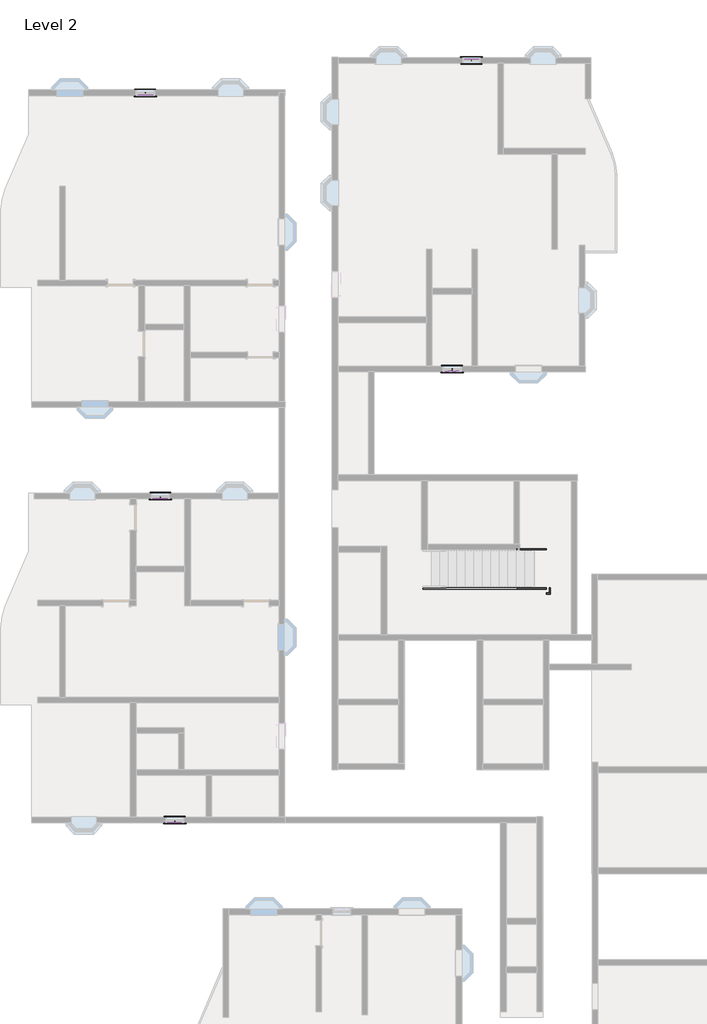
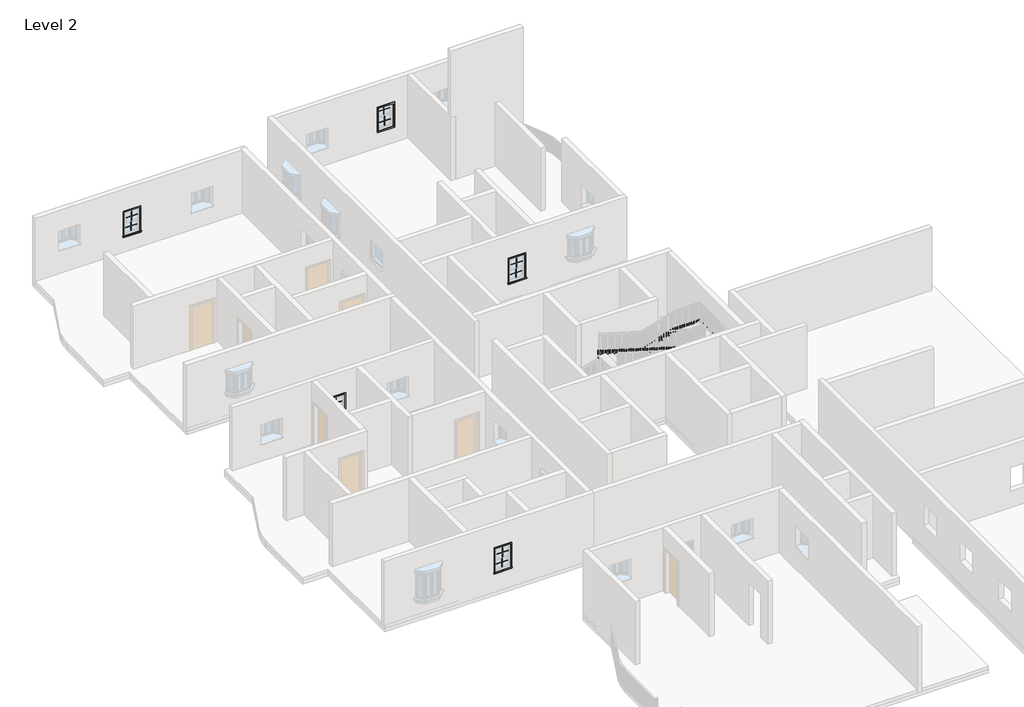
# One storey, part 14 of 14: 20 proxies, 6 members.
"""IFC4 building model written with IfcOpenShell, lengths in millimetres."""

from ifc_helpers import new_model, si_unit, frame, origin, place, context, project, spatial, polyline, outline, extrude, transform, mapped, element, save
from components import muntin_pattern_2x2_muntin_pattern_2x2_c35c595f, trim_window_exterior_flat_with_sill_e38017c9, trim_window_interior_flat_picture_frame_d728ed12

model = new_model("IFC4")

# Units and contexts
model_context = context("Model", 3, world=origin())
ifc_project = project(units=[si_unit("LENGTHUNIT", "METRE", prefix="MILLI")], contexts=[model_context])

# Site, building, storey
site = spatial("IfcSite", under=ifc_project)
building = spatial("IfcBuilding", under=site)
storey = spatial("IfcBuildingStorey", under=building, Name="Level 2", Elevation=3048.0)

# Proxies
placement = place(None, origin())
muntin_pattern_2x2_muntin_pattern_2x2_shape = muntin_pattern_2x2_muntin_pattern_2x2_c35c595f(model_context)
element("IfcBuildingElementProxy", 1, Name="Muntin Pattern_2x2 : Muntin Pattern_2x2", ObjectType="Muntin Pattern_2x2 : Muntin Pattern_2x2", at=placement, inside=storey, context=model_context, shape_type="MappedRepresentation", body=[
    mapped(muntin_pattern_2x2_muntin_pattern_2x2_shape, transform((-14639.3891351, 14368.0833494, 4518.025), x_axis=(-1.0, 0.0, 0.0), y_axis=(0.0, -1.0, 0.0), z_axis=(0.0, 0.0, 1.0))),
])
element("IfcBuildingElementProxy", 2, Name="Muntin Pattern_2x2 : Muntin Pattern_2x2", ObjectType="Muntin Pattern_2x2 : Muntin Pattern_2x2", at=placement, inside=storey, context=model_context, shape_type="MappedRepresentation", body=[
    mapped(muntin_pattern_2x2_muntin_pattern_2x2_shape, transform((-14639.3891351, 14412.5333494, 4038.6), x_axis=(-1.0, 0.0, 0.0), y_axis=(0.0, -1.0, 0.0), z_axis=(0.0, 0.0, 1.0))),
])
element("IfcBuildingElementProxy", 3, Name="Muntin Pattern_2x2 : Muntin Pattern_2x2", ObjectType="Muntin Pattern_2x2 : Muntin Pattern_2x2", at=placement, inside=storey, context=model_context, shape_type="MappedRepresentation", body=[
    mapped(muntin_pattern_2x2_muntin_pattern_2x2_shape, transform((-14125.0391351, 2785.6833494, 4518.025), x_axis=(-1.0, 0.0, 0.0), y_axis=(0.0, -1.0, 0.0), z_axis=(0.0, 0.0, 1.0))),
])
element("IfcBuildingElementProxy", 4, Name="Muntin Pattern_2x2 : Muntin Pattern_2x2", ObjectType="Muntin Pattern_2x2 : Muntin Pattern_2x2", at=placement, inside=storey, context=model_context, shape_type="MappedRepresentation", body=[
    mapped(muntin_pattern_2x2_muntin_pattern_2x2_shape, transform((-14125.0391351, 2830.1333494, 4038.6), x_axis=(-1.0, 0.0, 0.0), y_axis=(0.0, -1.0, 0.0), z_axis=(0.0, 0.0, 1.0))),
])
element("IfcBuildingElementProxy", 5, Name="Muntin Pattern_2x2 : Muntin Pattern_2x2", ObjectType="Muntin Pattern_2x2 : Muntin Pattern_2x2", at=placement, inside=storey, context=model_context, shape_type="MappedRepresentation", body=[
    mapped(muntin_pattern_2x2_muntin_pattern_2x2_shape, transform((-4206.3391351, 18910.0465905, 4518.025), x_axis=(-1.0, 0.0, 0.0), y_axis=(0.0, -1.0, 0.0), z_axis=(0.0, 0.0, 1.0))),
])
element("IfcBuildingElementProxy", 6, Name="Muntin Pattern_2x2 : Muntin Pattern_2x2", ObjectType="Muntin Pattern_2x2 : Muntin Pattern_2x2", at=placement, inside=storey, context=model_context, shape_type="MappedRepresentation", body=[
    mapped(muntin_pattern_2x2_muntin_pattern_2x2_shape, transform((-4206.3391351, 18954.4965905, 4038.6), x_axis=(-1.0, 0.0, 0.0), y_axis=(0.0, -1.0, 0.0), z_axis=(0.0, 0.0, 1.0))),
])
element("IfcBuildingElementProxy", 7, Name="Muntin Pattern_2x2 : Muntin Pattern_2x2", ObjectType="Muntin Pattern_2x2 : Muntin Pattern_2x2", at=placement, inside=storey, context=model_context, shape_type="MappedRepresentation", body=[
    mapped(muntin_pattern_2x2_muntin_pattern_2x2_shape, transform((-3514.1891351, 30066.9965905, 4518.025), x_axis=(1.0, 0.0, 0.0), y_axis=(0.0, 1.0, 0.0), z_axis=(0.0, 0.0, 1.0))),
])
element("IfcBuildingElementProxy", 8, Name="Muntin Pattern_2x2 : Muntin Pattern_2x2", ObjectType="Muntin Pattern_2x2 : Muntin Pattern_2x2", at=placement, inside=storey, context=model_context, shape_type="MappedRepresentation", body=[
    mapped(muntin_pattern_2x2_muntin_pattern_2x2_shape, transform((-3514.1891351, 30022.5465905, 4038.6), x_axis=(1.0, 0.0, 0.0), y_axis=(0.0, 1.0, 0.0), z_axis=(0.0, 0.0, 1.0))),
])
element("IfcBuildingElementProxy", 9, Name="Muntin Pattern_2x2 : Muntin Pattern_2x2", ObjectType="Muntin Pattern_2x2 : Muntin Pattern_2x2", at=placement, inside=storey, context=model_context, shape_type="MappedRepresentation", body=[
    mapped(muntin_pattern_2x2_muntin_pattern_2x2_shape, transform((-15175.9641351, 28782.5833494, 4518.025), x_axis=(-1.0, 0.0, 0.0), y_axis=(0.0, -1.0, 0.0), z_axis=(0.0, 0.0, 1.0))),
])
element("IfcBuildingElementProxy", 10, Name="Muntin Pattern_2x2 : Muntin Pattern_2x2", ObjectType="Muntin Pattern_2x2 : Muntin Pattern_2x2", at=placement, inside=storey, context=model_context, shape_type="MappedRepresentation", body=[
    mapped(muntin_pattern_2x2_muntin_pattern_2x2_shape, transform((-15175.9641351, 28827.0333494, 4038.6), x_axis=(-1.0, 0.0, 0.0), y_axis=(0.0, -1.0, 0.0), z_axis=(0.0, 0.0, 1.0))),
])
trim_window_exterior_flat_with_sill_shape = trim_window_exterior_flat_with_sill_e38017c9(model_context)
element("IfcBuildingElementProxy", 11, Name="Trim-Window-Exterior-Flat : with Sill", ObjectType="Trim-Window-Exterior-Flat : with Sill", at=placement, inside=storey, context=model_context, shape_type="MappedRepresentation", body=[
    mapped(trim_window_exterior_flat_with_sill_shape, transform((-14639.3891351, 14333.1583494, 5029.2), x_axis=(1.0, 0.0, 0.0), y_axis=(0.0, 0.0, 1.0), z_axis=(0.0, -1.0, 0.0))),
])
element("IfcBuildingElementProxy", 12, Name="Trim-Window-Exterior-Flat : with Sill", ObjectType="Trim-Window-Exterior-Flat : with Sill", at=placement, inside=storey, context=model_context, shape_type="MappedRepresentation", body=[
    mapped(trim_window_exterior_flat_with_sill_shape, transform((-14125.0391351, 2750.7583494, 5029.2), x_axis=(1.0, 0.0, 0.0), y_axis=(0.0, 0.0, 1.0), z_axis=(0.0, -1.0, 0.0))),
])
element("IfcBuildingElementProxy", 13, Name="Trim-Window-Exterior-Flat : with Sill", ObjectType="Trim-Window-Exterior-Flat : with Sill", at=placement, inside=storey, context=model_context, shape_type="MappedRepresentation", body=[
    mapped(trim_window_exterior_flat_with_sill_shape, transform((-4206.3391351, 18875.1215905, 5029.2), x_axis=(1.0, 0.0, 0.0), y_axis=(0.0, 0.0, 1.0), z_axis=(0.0, -1.0, 0.0))),
])
element("IfcBuildingElementProxy", 14, Name="Trim-Window-Exterior-Flat : with Sill", ObjectType="Trim-Window-Exterior-Flat : with Sill", at=placement, inside=storey, context=model_context, shape_type="MappedRepresentation", body=[
    mapped(trim_window_exterior_flat_with_sill_shape, transform((-3514.1891351, 30101.9215905, 5029.2), x_axis=(-1.0, 0.0, 0.0), y_axis=(0.0, 0.0, 1.0), z_axis=(0.0, 1.0, 0.0))),
])
element("IfcBuildingElementProxy", 15, Name="Trim-Window-Exterior-Flat : with Sill", ObjectType="Trim-Window-Exterior-Flat : with Sill", at=placement, inside=storey, context=model_context, shape_type="MappedRepresentation", body=[
    mapped(trim_window_exterior_flat_with_sill_shape, transform((-15175.9641351, 28747.6583494, 5029.2), x_axis=(1.0, 0.0, 0.0), y_axis=(0.0, 0.0, 1.0), z_axis=(0.0, -1.0, 0.0))),
])
trim_window_interior_flat_picture_frame_shape = trim_window_interior_flat_picture_frame_d728ed12(model_context)
element("IfcBuildingElementProxy", 16, Name="Trim-Window-Interior-Flat : Picture Frame", ObjectType="Trim-Window-Interior-Flat : Picture Frame", at=placement, inside=storey, context=model_context, shape_type="MappedRepresentation", body=[
    mapped(trim_window_interior_flat_picture_frame_shape, transform((-14639.3891351, 14536.3583494, 5029.2), x_axis=(-1.0, 0.0, 0.0), y_axis=(0.0, 0.0, 1.0), z_axis=(0.0, 1.0, 0.0))),
])
element("IfcBuildingElementProxy", 17, Name="Trim-Window-Interior-Flat : Picture Frame", ObjectType="Trim-Window-Interior-Flat : Picture Frame", at=placement, inside=storey, context=model_context, shape_type="MappedRepresentation", body=[
    mapped(trim_window_interior_flat_picture_frame_shape, transform((-14125.0391351, 2953.9583494, 5029.2), x_axis=(-1.0, 0.0, 0.0), y_axis=(0.0, 0.0, 1.0), z_axis=(0.0, 1.0, 0.0))),
])
element("IfcBuildingElementProxy", 18, Name="Trim-Window-Interior-Flat : Picture Frame", ObjectType="Trim-Window-Interior-Flat : Picture Frame", at=placement, inside=storey, context=model_context, shape_type="MappedRepresentation", body=[
    mapped(trim_window_interior_flat_picture_frame_shape, transform((-4206.3391351, 19078.3215905, 5029.2), x_axis=(-1.0, 0.0, 0.0), y_axis=(0.0, 0.0, 1.0), z_axis=(0.0, 1.0, 0.0))),
])
element("IfcBuildingElementProxy", 19, Name="Trim-Window-Interior-Flat : Picture Frame", ObjectType="Trim-Window-Interior-Flat : Picture Frame", at=placement, inside=storey, context=model_context, shape_type="MappedRepresentation", body=[
    mapped(trim_window_interior_flat_picture_frame_shape, transform((-3514.1891351, 29898.7215905, 5029.2), x_axis=(1.0, 0.0, 0.0), y_axis=(0.0, 0.0, 1.0), z_axis=(0.0, -1.0, 0.0))),
])
element("IfcBuildingElementProxy", 20, Name="Trim-Window-Interior-Flat : Picture Frame", ObjectType="Trim-Window-Interior-Flat : Picture Frame", at=placement, inside=storey, context=model_context, shape_type="MappedRepresentation", body=[
    mapped(trim_window_interior_flat_picture_frame_shape, transform((-15175.9641351, 28950.8583494, 5029.2), x_axis=(-1.0, 0.0, 0.0), y_axis=(0.0, 0.0, 1.0), z_axis=(0.0, 1.0, 0.0))),
])

# Members
element("IfcMember", 21, ObjectType="Stringer - 2\" Width", at=placement, inside=storey, context=model_context, shape_type="SweptSolid", body=[
    extrude(outline(polyline([(3239.5995961, -5254.0891351), (3048.0, -5254.0891351), (3048.0, -4832.019314), (4495.8, -6.019314), (4495.8, -1066.7544553), (3239.5995961, -5254.0891351)])), frame((0.0, 12506.0715905, 0.0), z_axis=(0.0, 1.0, 0.0), x_axis=(0.0, 0.0, 1.0)), (0.0, 0.0, 1.0), 50.8),
])
element("IfcMember", 22, ObjectType="Stringer - 2\" Width", at=placement, inside=storey, context=model_context, shape_type="SweptSolid", body=[
    extrude(outline(polyline([(54.5108649, 12556.8715905), (105.3108649, 12556.8715905), (105.3108649, 9478.4949943), (54.5108649, 9478.4949943), (54.5108649, 12556.8715905)])), frame((0.0, 0.0, 4191.0), z_axis=(0.0, 0.0, 1.0), x_axis=(1.0, 0.0, 0.0)), (0.0, 0.0, 1.0), 304.8),
])
element("IfcMember", 23, ObjectType="Stringer - 2\" Width", at=placement, inside=storey, context=model_context, shape_type="SweptSolid", body=[
    extrude(outline(polyline([(4191.0, 105.3108649), (4283.5395961, 105.3108649), (5891.3595961, -5254.0891351), (5573.1390537, -5254.0891351), (4191.0, -646.9589562), (4191.0, 105.3108649)])), frame((0.0, 9427.6949943, 0.0), z_axis=(0.0, 1.0, 0.0), x_axis=(0.0, 0.0, 1.0)), (0.0, 0.0, 1.0), 50.8),
])
element("IfcMember", 24, ObjectType="Stringer - 2\" Width", at=placement, inside=storey, context=model_context, shape_type="SweptSolid", body=[
    extrude(outline(polyline([(3239.5995961, -5254.0891351), (3048.0, -5254.0891351), (3048.0, -4832.019314), (4277.7390537, -732.8891351), (4495.8, -732.8891351), (4495.8, -1066.7544553), (3239.5995961, -5254.0891351)])), frame((0.0, 11103.4082924, 0.0), z_axis=(0.0, 1.0, 0.0), x_axis=(0.0, 0.0, 1.0)), (0.0, 0.0, 1.0), 50.8),
])
element("IfcMember", 25, ObjectType="Stringer - 2\" Width", at=placement, inside=storey, context=model_context, shape_type="SweptSolid", body=[
    extrude(outline(polyline([(-732.8891351, 11154.2082924), (-682.0891351, 11154.2082924), (-682.0891351, 10976.4082924), (-732.8891351, 10976.4082924), (-732.8891351, 11154.2082924)])), frame((0.0, 0.0, 4191.0), z_axis=(0.0, 0.0, 1.0), x_axis=(1.0, 0.0, 0.0)), (0.0, 0.0, 1.0), 304.8),
])
element("IfcMember", 26, ObjectType="Stringer - 2\" Width", at=placement, inside=storey, context=model_context, shape_type="SweptSolid", body=[
    extrude(outline(polyline([(4201.5390537, -682.0891351), (4519.7595961, -682.0891351), (5891.3595961, -5254.0891351), (5573.1390537, -5254.0891351), (4201.5390537, -682.0891351)])), frame((0.0, 10925.6082924, 0.0), z_axis=(0.0, 1.0, 0.0), x_axis=(0.0, 0.0, 1.0)), (0.0, 0.0, 1.0), 50.8),
])

save(model, "model.ifc")

# Revit data of these elements
# Type "Muntin Pattern_2x2 : Muntin Pattern_2x2"
#   Width [instance default] = 4' - 0"
#   Thickness = 0' - 0 1/2"
#   Height [instance default] = 4' - 0"
#   Distance = 0' - 0 3/4"
#   Interior Material [instance default] = none
#   Exterior Material [instance default] = none
#   Default Elevation = 0
# Type "Trim-Window-Exterior-Flat : with Sill"
#   Trim Width = 0' - 2 1/4"
#   Trim Thickness_Picture Frame = 0' - 1 1/4"
#   Trim Thickness_with Sill = 0' - 0 3/4"
#   Sill Thickness = 0' - 1 1/4"
#   Opening Width [instance default] = 2' - 0"
#   Opening Height [instance default] = 3' - 0"
#   Default Elevation = 4' - 0"
#   Sill = yes
#   Picture Frame = no
#   Trim Material [instance default] = none
# Type "Trim-Window-Interior-Flat : Picture Frame"
#   Trim Thickness_Picture Frame = 0' - 1 1/4"
#   Trim Width = 0' - 2 1/4"
#   Trim Thickness_with Sill = 0' - 0 3/4"
#   Sill Thickness = 0' - 1 1/4"
#   Opening Width [instance default] = 2' - 0"
#   Opening Height [instance default] = 3' - 0"
#   Default Elevation = 4' - 0"
#   Sill = no
#   Picture Frame = yes
#   Trim Material [instance default] = none
# Elements 1, 2, 3, 4, 5, 6, 7, 8, 9, 10 (IfcBuildingElementProxy, "Muntin Pattern_2x2 : Muntin Pattern_2x2")
#   Width = 1' - 8"
#   Height = 1' - 5 1/8"
#   Interior Material = Wood - Stained
#   Exterior Material = Clad - White
#   Phase Created = New Construction
#   Materials on its faces: "Clad - White", "Wood - Stained"
# Elements 11, 12, 13, 14, 15 (IfcBuildingElementProxy, "Trim-Window-Exterior-Flat : with Sill")
#   Opening Width = 2' - 2"
#   Opening Height = 3' - 6"
#   Trim Material = Clad - White
#   Phase Created = New Construction
#   Materials on its faces: "Clad - White"
# Elements 16, 17, 18, 19, 20 (IfcBuildingElementProxy, "Trim-Window-Interior-Flat : Picture Frame")
#   Opening Width = 2' - 2"
#   Opening Height = 3' - 6"
#   Trim Material = Wood - Stained
#   Phase Created = New Construction
#   Materials on its faces: "Wood - Stained"
# Elements 21, 22, 23, 24, 25, 26 (IfcMember, "Stringer - 2\" Width")
#   Phase Created = New Construction
# Materials
#   "Clad - White": class "Wood", colour RGB 242 242 238, transparency 0, Cost = 0
#   "Wood - Stained": class "Wood", colour RGB 224 178 126, transparency 0, Cost = 0
